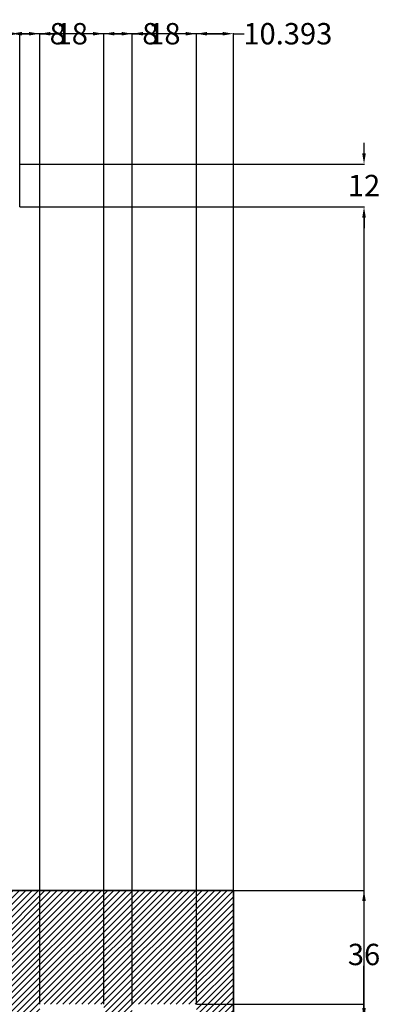
# Model space of a CAD drawing. Units: inches. Extents: x 126 to 726, y 86 to 888.
# Tile 13 of 13: x 606 to 709, y 611 to 888. Entities that reach past the tile are written whole.
import ezdxf

# ---------------------------------------------------------------- set-up
doc = ezdxf.new("R2010")
doc.units = ezdxf.units.IN
doc.header["$MEASUREMENT"] = 0
for name, color, linetype, lineweight in [('A-ANNO-DIMS', 2, 'Continuous', 18), ('A-ELEV', 7, 'Continuous', 35), ('A-ELEV-PATT', 8, 'Continuous', 13)]:
    doc.layers.add(name, color=color, linetype=linetype, lineweight=lineweight)
doc.styles.get("Standard").update_dxf_attribs({"font": 'arial.ttf'})
doc.dimstyles.get("Standard").update_dxf_attribs({"dimtxt": 6, "dimasz": 3, "dimexe": 0.18, "dimexo": 0.0625, "dimgap": 0.09, "dimtad": 0, "dimtih": 1, "dimtoh": 1, "dimdec": 0, "dimzin": 0, "dimdsep": 46, "dimlunit": 3, "dimtxsty": 'Standard', "dimcen": 0.09, "dimadec": 0, "dimazin": 0, "dimtfac": 1, "dimtdec": 0, "dimtofl": 0, "dimtmove": 0, "dimatfit": 3, "dimfxl": 1, "dimtolj": 1, "dimtzin": 0, "dimarcsym": 0})

# ---------------------------------------------------------------- blocks, each defined once
blk = doc.blocks.new('*D13')
at = {"layer": 'A-ANNO-DIMS', "color": 0, "lineweight": -2, "transparency": 16777216}
for p, q in [((665.97, 642.98), (665.97, 90.21)), ((185.97, 126.98), (185.97, 90.21)), ((188.97, 90.39), (419.15, 90.39)), ((662.97, 90.39), (432.8, 90.39))]:
    blk.add_line(p, q, dxfattribs=at)
at = {"layer": 'A-ANNO-DIMS', "color": 0, "transparency": 16777216}
for points in [[(188.97, 90.89), (188.97, 89.89), (185.97, 90.39)], [(662.97, 90.89), (662.97, 89.89), (665.97, 90.39)]]:
    blk.add_solid(points, dxfattribs=at)
at = {"layer": 'Defpoints', "color": 0, "transparency": 16777216}
for p in [(665.97, 643.04), (185.97, 127.04), (665.97, 90.39)]:
    blk.add_point(p, dxfattribs=at)
at = {"layer": 'A-ANNO-DIMS', "color": 0, "transparency": 16777216, "insert": (425.97, 90.39), "char_height": 6, "attachment_point": 5}
blk.add_mtext('\\A1;480', dxfattribs=at)
blk = doc.blocks.new('*D26')
at = {"layer": 'A-ANNO-DIMS', "color": 0, "lineweight": -2, "transparency": 16777216}
for p, q in [((485.97, 835.1), (485.97, 883.87)), ((488.97, 883.69), (539.55, 883.69)), ((602.97, 883.69), (552.4, 883.69)), ((605.97, 835.1), (605.97, 883.87))]:
    blk.add_line(p, q, dxfattribs=at)
at = {"layer": 'A-ANNO-DIMS', "color": 0, "transparency": 16777216}
for points in [[(488.97, 884.19), (488.97, 883.19), (485.97, 883.69)], [(602.97, 884.19), (602.97, 883.19), (605.97, 883.69)]]:
    blk.add_solid(points, dxfattribs=at)
at = {"layer": 'Defpoints', "color": 0, "transparency": 16777216}
for p in [(605.97, 883.69), (485.97, 835.04), (605.97, 835.04)]:
    blk.add_point(p, dxfattribs=at)
at = {"layer": 'A-ANNO-DIMS', "color": 0, "transparency": 16777216, "insert": (545.97, 883.69), "char_height": 6, "attachment_point": 5}
blk.add_mtext('\\A1;120', dxfattribs=at)
blk = doc.blocks.new('*D27')
at = {"layer": 'A-ANNO-DIMS', "color": 0, "lineweight": -2, "transparency": 16777216}
for p, q in [((702.624909, 850.042369), (702.624909, 853.042369)), ((606.037409, 847.042369), (702.804909, 847.042369)), ((606.037409, 835.042369), (702.804909, 835.042369)), ((702.624909, 832.042369), (702.624909, 829.042369))]:
    blk.add_line(p, q, dxfattribs=at)
at = {"layer": 'A-ANNO-DIMS', "color": 0, "transparency": 16777216}
for points in [[(702.124909, 850.042369), (703.124909, 850.042369), (702.624909, 847.042369)], [(702.124909, 832.042369), (703.124909, 832.042369), (702.624909, 835.042369)]]:
    blk.add_solid(points, dxfattribs=at)
at = {"layer": 'Defpoints', "color": 0, "transparency": 16777216}
for p in [(605.974909, 847.042369), (702.624909, 847.042369), (605.974909, 835.042369)]:
    blk.add_point(p, dxfattribs=at)
at = {"layer": 'A-ANNO-DIMS', "color": 0, "transparency": 16777216, "insert": (702.624909, 841.042369), "char_height": 6, "attachment_point": 5}
blk.add_mtext('\\A1;12', dxfattribs=at)
blk = doc.blocks.new('*D29')
at = {"layer": 'A-ANNO-DIMS', "color": 0, "lineweight": -2, "transparency": 16777216}
for p, q in [((606.04, 835.04), (702.8, 835.04)), ((702.62, 832.04), (702.62, 598.2)), ((702.62, 358.04), (702.62, 591.89)), ((666.04, 355.04), (702.8, 355.04))]:
    blk.add_line(p, q, dxfattribs=at)
at = {"layer": 'A-ANNO-DIMS', "color": 0, "transparency": 16777216}
for points in [[(702.12, 832.04), (703.12, 832.04), (702.62, 835.04)], [(702.12, 358.04), (703.12, 358.04), (702.62, 355.04)]]:
    blk.add_solid(points, dxfattribs=at)
at = {"layer": 'Defpoints', "color": 0, "transparency": 16777216}
for p in [(605.97, 835.04), (702.62, 835.04), (665.97, 355.04)]:
    blk.add_point(p, dxfattribs=at)
at = {"layer": 'A-ANNO-DIMS', "color": 0, "transparency": 16777216, "insert": (702.62, 595.04), "char_height": 6, "attachment_point": 5}
blk.add_mtext('\\A1;480', dxfattribs=at)
blk = doc.blocks.new('*D41')
at = {"layer": 'A-ANNO-DIMS', "color": 0, "lineweight": -2, "transparency": 16777216}
for p, q in [((429.97, 607.1), (429.97, 883.87)), ((432.97, 883.69), (541.21, 883.69)), ((662.97, 883.69), (554.74, 883.69)), ((665.97, 607.1), (665.97, 883.87))]:
    blk.add_line(p, q, dxfattribs=at)
at = {"layer": 'A-ANNO-DIMS', "color": 0, "transparency": 16777216}
for points in [[(432.97, 884.19), (432.97, 883.19), (429.97, 883.69)], [(662.97, 884.19), (662.97, 883.19), (665.97, 883.69)]]:
    blk.add_solid(points, dxfattribs=at)
at = {"layer": 'Defpoints', "color": 0, "transparency": 16777216}
for p in [(665.97, 883.69), (429.97, 607.04), (665.97, 607.04)]:
    blk.add_point(p, dxfattribs=at)
at = {"layer": 'A-ANNO-DIMS', "color": 0, "transparency": 16777216, "insert": (547.97, 883.69), "char_height": 6, "attachment_point": 5}
blk.add_mtext('\\A1;236', dxfattribs=at)
blk = doc.blocks.new('*D48')
at = {"layer": 'A-ANNO-DIMS', "color": 0, "lineweight": -2, "transparency": 16777216}
for p, q in [((702.624909, 610.042369), (702.624909, 613.042369)), ((666.037409, 607.042369), (702.804909, 607.042369)), ((666.037409, 595.042369), (702.804909, 595.042369)), ((702.624909, 592.042369), (702.624909, 589.042369))]:
    blk.add_line(p, q, dxfattribs=at)
at = {"layer": 'A-ANNO-DIMS', "color": 0, "transparency": 16777216}
for points in [[(702.124909, 610.042369), (703.124909, 610.042369), (702.624909, 607.042369)], [(702.124909, 592.042369), (703.124909, 592.042369), (702.624909, 595.042369)]]:
    blk.add_solid(points, dxfattribs=at)
at = {"layer": 'Defpoints', "color": 0, "transparency": 16777216}
for p in [(665.974909, 607.042369), (702.624909, 607.042369), (665.974909, 595.042369)]:
    blk.add_point(p, dxfattribs=at)
at = {"layer": 'A-ANNO-DIMS', "color": 0, "transparency": 16777216, "insert": (702.624909, 601.042369), "char_height": 6, "attachment_point": 5}
blk.add_mtext('\\A1;12', dxfattribs=at)
blk = doc.blocks.new('*D49')
at = {"layer": 'A-ANNO-DIMS', "color": 0, "lineweight": -2, "transparency": 16777216}
for p, q in [((666.04, 643.04), (702.8, 643.04)), ((702.62, 640.04), (702.62, 628.2)), ((702.62, 610.04), (702.62, 621.89)), ((666.04, 607.04), (702.8, 607.04))]:
    blk.add_line(p, q, dxfattribs=at)
at = {"layer": 'A-ANNO-DIMS', "color": 0, "transparency": 16777216}
for points in [[(702.12, 640.04), (703.12, 640.04), (702.62, 643.04)], [(702.12, 610.04), (703.12, 610.04), (702.62, 607.04)]]:
    blk.add_solid(points, dxfattribs=at)
at = {"layer": 'Defpoints', "color": 0, "transparency": 16777216}
for p in [(665.97, 643.04), (702.62, 643.04), (665.97, 607.04)]:
    blk.add_point(p, dxfattribs=at)
at = {"layer": 'A-ANNO-DIMS', "color": 0, "transparency": 16777216, "insert": (702.62, 625.04), "char_height": 6, "attachment_point": 5}
blk.add_mtext('\\A1;36', dxfattribs=at)
blk = doc.blocks.new('*D52')
at = {"layer": 'A-ANNO-DIMS', "color": 0, "lineweight": -2, "transparency": 16777216}
for p, q in [((603.58, 611.1), (603.58, 883.87)), ((606.58, 883.69), (608.58, 883.69)), ((611.58, 611.1), (611.58, 883.87)), ((611.58, 883.69), (614.58, 883.69))]:
    blk.add_line(p, q, dxfattribs=at)
at = {"layer": 'A-ANNO-DIMS', "color": 0, "transparency": 16777216}
for points in [[(606.58, 884.19), (606.58, 883.19), (603.58, 883.69)], [(608.58, 884.19), (608.58, 883.19), (611.58, 883.69)]]:
    blk.add_solid(points, dxfattribs=at)
at = {"layer": 'Defpoints', "color": 0, "transparency": 16777216}
for p in [(611.58, 883.69), (603.58, 611.04), (611.58, 611.04)]:
    blk.add_point(p, dxfattribs=at)
at = {"layer": 'A-ANNO-DIMS', "color": 0, "transparency": 16777216, "insert": (616.65, 883.69), "char_height": 6, "attachment_point": 5}
blk.add_mtext('\\A1;8', dxfattribs=at)
blk = doc.blocks.new('*D53')
at = {"layer": 'A-ANNO-DIMS', "color": 0, "lineweight": -2, "transparency": 16777216}
for p, q in [((611.58, 611.1), (611.58, 883.87)), ((614.58, 883.69), (616.47, 883.69)), ((626.58, 883.69), (624.69, 883.69)), ((629.58, 611.1), (629.58, 883.87))]:
    blk.add_line(p, q, dxfattribs=at)
at = {"layer": 'A-ANNO-DIMS', "color": 0, "transparency": 16777216}
for points in [[(614.58, 884.19), (614.58, 883.19), (611.58, 883.69)], [(626.58, 884.19), (626.58, 883.19), (629.58, 883.69)]]:
    blk.add_solid(points, dxfattribs=at)
at = {"layer": 'Defpoints', "color": 0, "transparency": 16777216}
for p in [(629.58, 883.69), (611.58, 611.04), (629.58, 611.04)]:
    blk.add_point(p, dxfattribs=at)
at = {"layer": 'A-ANNO-DIMS', "color": 0, "transparency": 16777216, "insert": (620.58, 883.69), "char_height": 6, "attachment_point": 5}
blk.add_mtext('\\A1;18', dxfattribs=at)
blk = doc.blocks.new('*D54')
at = {"layer": 'A-ANNO-DIMS', "color": 0, "lineweight": -2, "transparency": 16777216}
for p, q in [((629.58, 611.1), (629.58, 883.87)), ((632.58, 883.69), (634.58, 883.69)), ((637.58, 611.1), (637.58, 883.87)), ((637.58, 883.69), (640.58, 883.69))]:
    blk.add_line(p, q, dxfattribs=at)
at = {"layer": 'A-ANNO-DIMS', "color": 0, "transparency": 16777216}
for points in [[(632.58, 884.19), (632.58, 883.19), (629.58, 883.69)], [(634.58, 884.19), (634.58, 883.19), (637.58, 883.69)]]:
    blk.add_solid(points, dxfattribs=at)
at = {"layer": 'Defpoints', "color": 0, "transparency": 16777216}
for p in [(637.58, 883.69), (629.58, 611.04), (637.58, 611.04)]:
    blk.add_point(p, dxfattribs=at)
at = {"layer": 'A-ANNO-DIMS', "color": 0, "transparency": 16777216, "insert": (642.65, 883.69), "char_height": 6, "attachment_point": 5}
blk.add_mtext('\\A1;8', dxfattribs=at)
blk = doc.blocks.new('*D55')
at = {"layer": 'A-ANNO-DIMS', "color": 0, "lineweight": -2, "transparency": 16777216}
for p, q in [((637.58, 611.1), (637.58, 883.87)), ((640.58, 883.69), (642.47, 883.69)), ((652.58, 883.69), (650.69, 883.69)), ((655.58, 611.1), (655.58, 883.87))]:
    blk.add_line(p, q, dxfattribs=at)
at = {"layer": 'A-ANNO-DIMS', "color": 0, "transparency": 16777216}
for points in [[(640.58, 884.19), (640.58, 883.19), (637.58, 883.69)], [(652.58, 884.19), (652.58, 883.19), (655.58, 883.69)]]:
    blk.add_solid(points, dxfattribs=at)
at = {"layer": 'Defpoints', "color": 0, "transparency": 16777216}
for p in [(655.58, 883.69), (637.58, 611.04), (655.58, 611.04)]:
    blk.add_point(p, dxfattribs=at)
at = {"layer": 'A-ANNO-DIMS', "color": 0, "transparency": 16777216, "insert": (646.58, 883.69), "char_height": 6, "attachment_point": 5}
blk.add_mtext('\\A1;18', dxfattribs=at)
blk = doc.blocks.new('*D56')
at = {"layer": 'A-ANNO-DIMS', "color": 0, "lineweight": -2, "transparency": 16777216}
for p, q in [((655.58, 611.1), (655.58, 883.87)), ((658.58, 883.69), (662.97, 883.69)), ((665.97, 643.1), (665.97, 883.87)), ((665.97, 883.69), (668.97, 883.69))]:
    blk.add_line(p, q, dxfattribs=at)
at = {"layer": 'A-ANNO-DIMS', "color": 0, "transparency": 16777216}
for points in [[(658.58, 884.19), (658.58, 883.19), (655.58, 883.69)], [(662.97, 884.19), (662.97, 883.19), (665.97, 883.69)]]:
    blk.add_solid(points, dxfattribs=at)
at = {"layer": 'Defpoints', "color": 0, "transparency": 16777216}
for p in [(665.97, 883.69), (665.97, 643.04), (655.58, 611.04)]:
    blk.add_point(p, dxfattribs=at)
at = {"layer": 'A-ANNO-DIMS', "color": 0, "transparency": 16777216, "insert": (681.24, 883.69), "char_height": 6, "attachment_point": 5}
blk.add_mtext('\\A1;10.393', dxfattribs=at)
blk = doc.blocks.new('*D57')
at = {"layer": 'A-ANNO-DIMS', "color": 0, "lineweight": -2, "transparency": 16777216}
for p, q in [((655.64, 611.04), (702.8, 611.04)), ((702.62, 608.04), (702.62, 486.2)), ((702.62, 358.04), (702.62, 479.89)), ((655.64, 355.04), (702.8, 355.04))]:
    blk.add_line(p, q, dxfattribs=at)
at = {"layer": 'A-ANNO-DIMS', "color": 0, "transparency": 16777216}
for points in [[(702.12, 608.04), (703.12, 608.04), (702.62, 611.04)], [(702.12, 358.04), (703.12, 358.04), (702.62, 355.04)]]:
    blk.add_solid(points, dxfattribs=at)
at = {"layer": 'Defpoints', "color": 0, "transparency": 16777216}
for p in [(655.58, 611.04), (702.62, 611.04), (655.58, 355.04)]:
    blk.add_point(p, dxfattribs=at)
at = {"layer": 'A-ANNO-DIMS', "color": 0, "transparency": 16777216, "insert": (702.62, 483.04), "char_height": 6, "attachment_point": 5}
blk.add_mtext('\\A1;256', dxfattribs=at)

msp = doc.modelspace()

# ---------------------------------------------------------------- hatches: boundary and pattern name
at = {"layer": 'A-ELEV-PATT'}
h = msp.add_hatch(dxfattribs=at)
h.set_pattern_fill('ANSI31', color=256, scale=10)
h.paths.add_polyline_path([(585.5818, 607.0424), (585.5818, 611.0424), (603.5818, 611.0424), (603.5818, 607.0424), (611.5818, 607.0424), (611.5818, 611.0424), (629.5818, 611.0424), (629.5818, 607.0424), (637.5818, 607.0424), (637.5818, 611.0424), (655.5818, 611.0424), (655.5818, 607.0424), (665.9749, 607.0424), (665.9749, 643.0424), (485.9749, 643.0424), (485.9749, 607.0424)])

# ---------------------------------------------------------------- linework, layer by layer
at = {"layer": 'A-ELEV'}
for p in [(485.9749, 643.0424), (665.9749, 595.0424)]:
    msp.add_line(p, (665.9749, 643.0424), dxfattribs=at)

# ---------------------------------------------------------------- dimensions: what is measured, and where the dimension line sits
at = {"layer": 'A-ANNO-DIMS'}
for base, p1, p2, override, picture, middle in [((665.9749, 883.6924), (429.9749, 607.0424), (665.9749, 607.0424), {"dimdec": 0, "dimlfac": 1, "dimrnd": 0, "dimzin": 0, "dimdsep": 46, "dimlunit": 2}, '*D41', (547.9749, 883.6924)), ((605.9749, 883.6924), (485.9749, 835.0424), (605.9749, 835.0424), {"dimdec": 0, "dimlfac": 1, "dimrnd": 0, "dimzin": 0, "dimdsep": 46, "dimlunit": 2}, '*D26', (545.9749, 883.6924)), ((611.5818, 883.6924), (603.5818, 611.0424), (611.5818, 611.0424), {"dimdec": 0, "dimlfac": 1, "dimrnd": 0, "dimzin": 0, "dimdsep": 46, "dimlunit": 2}, '*D52', (616.6486, 883.6924)), ((629.5818, 883.6924), (611.5818, 611.0424), (629.5818, 611.0424), {"dimdec": 0, "dimlfac": 1, "dimrnd": 0, "dimzin": 0, "dimdsep": 46, "dimlunit": 2}, '*D53', (620.5818, 883.6924)), ((637.5818, 883.6924), (629.5818, 611.0424), (637.5818, 611.0424), {"dimdec": 0, "dimlfac": 1, "dimrnd": 0, "dimzin": 0, "dimdsep": 46, "dimlunit": 2}, '*D54', (642.6486, 883.6924)), ((655.5818, 883.6924), (637.5818, 611.0424), (655.5818, 611.0424), {"dimdec": 0, "dimlfac": 1, "dimrnd": 0, "dimzin": 0, "dimdsep": 46, "dimlunit": 2}, '*D55', (646.5818, 883.6924)), ((665.9749, 883.6924), (655.5818, 611.0424), (665.9749, 643.0424), {"dimdec": 3, "dimlfac": 1, "dimrnd": 0, "dimzin": 0, "dimdsep": 46, "dimlunit": 2}, '*D56', (681.2368, 883.6924)), ((665.9749, 90.3924), (185.9749, 127.0424), (665.9749, 643.0424), {"dimdec": 0, "dimlfac": 1, "dimrnd": 0, "dimzin": 0, "dimdsep": 46, "dimlunit": 2}, '*D13', (425.9749, 90.3924))]:
    dim = msp.add_linear_dim(base=base, p1=p1, p2=p2, dimstyle='Standard', override=override, dxfattribs=at)
    dim.commit()
    dim.dimension.update_dxf_attribs({"geometry": picture, "text_midpoint": middle})
for base, p1, p2, picture, middle in [((702.6249, 847.0424), (605.9749, 835.0424), (605.9749, 847.0424), '*D27', (702.6249, 841.0424)), ((702.6249, 835.0424), (665.9749, 355.0424), (605.9749, 835.0424), '*D29', (702.6249, 595.0424)), ((702.6249, 643.0424), (665.9749, 607.0424), (665.9749, 643.0424), '*D49', (702.6249, 625.0424)), ((702.6249, 607.0424), (665.9749, 595.0424), (665.9749, 607.0424), '*D48', (702.6249, 601.0424)), ((702.6249, 611.0424), (655.5818, 355.0424), (655.5818, 611.0424), '*D57', (702.6249, 483.0424))]:
    dim = msp.add_linear_dim(base=base, p1=p1, p2=p2, angle=90, dimstyle='Standard', override={"dimdec": 0, "dimlfac": 1, "dimrnd": 0, "dimzin": 0, "dimdsep": 46, "dimlunit": 2}, dxfattribs=at)
    dim.commit()
    dim.dimension.update_dxf_attribs({"geometry": picture, "text_midpoint": middle})

doc.saveas('drawing.dxf')
